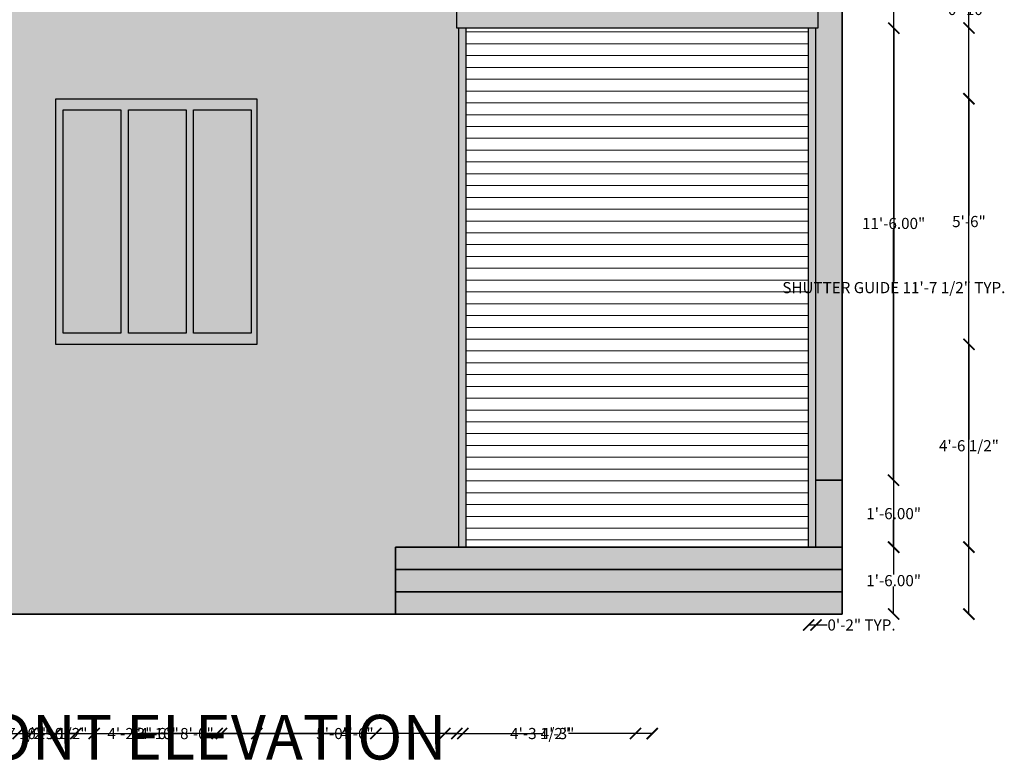
# Model space of a CAD drawing. Units: inches. Extents: x -654 to 390, y -40 to 648.
# Tile 4 of 13: x 126 to 390, y -40 to 159. Entities that reach past the tile are written whole.
import ezdxf

# ---------------------------------------------------------------- set-up
doc = ezdxf.new("R2010")
doc.units = ezdxf.units.IN
doc.header["$PDMODE"] = 3
for name, color, linetype, lineweight in [('A-ANNO-DIMS', 2, 'Continuous', 18), ('A-ANNO-TEXT', 7, 'Continuous', 25), ('A-DOOR', 3, 'Continuous', 25), ('A-ELEV', 7, 'Continuous', 35), ('A-ELEV-FILL', 252, 'Continuous', 13), ('A-ELEV-PATT', 8, 'Continuous', 13), ('A-GLAZ', 4, 'Continuous', 25)]:
    doc.layers.add(name, color=color, linetype=linetype, lineweight=lineweight)
doc.styles.get("Standard").update_dxf_attribs({"font": 'arial.ttf'})
doc.dimstyles.get("Standard").update_dxf_attribs({"dimtxt": 3, "dimasz": 3, "dimexe": 0.18, "dimexo": 0.0625, "dimgap": 0.09, "dimtad": 0, "dimtih": 1, "dimtoh": 1, "dimzin": 0, "dimdsep": 46, "dimlunit": 3, "dimtxsty": 'Standard', "dimblk": 'ARCHTICK', "dimcen": 0.09, "dimse1": 1, "dimse2": 1, "dimadec": 0, "dimazin": 0, "dimtfac": 1, "dimtofl": 0, "dimtmove": 0, "dimatfit": 3, "dimfxl": 1, "dimtolj": 1, "dimtzin": 0, "dimarcsym": 0})

# ---------------------------------------------------------------- blocks, each defined once
blk = doc.blocks.new('_ArchTick')
at = {"color": 0, "linetype": 'ByBlock', "const_width": 0.15}
blk.add_lwpolyline([(-0.5, -0.5), (0.5, 0.5)], dxfattribs=at)
blk = doc.blocks.new('*D2')
at = {"layer": 'A-ANNO-DIMS', "color": 0, "lineweight": -2, "transparency": 16777216}
for p, q in [((360.51, 17.13), (360.51, 9.76)), ((360.51, -0.87), (360.51, 6.51))]:
    blk.add_line(p, q, dxfattribs=at)
at = {"layer": 'Defpoints', "color": 0, "transparency": 16777216}
for p in [(346.65, 17.13), (360.51, 17.13), (346.65, -0.87)]:
    blk.add_point(p, dxfattribs=at)
at = {"layer": 'A-ANNO-DIMS', "color": 0, "lineweight": -2, "transparency": 16777216, "xscale": 3, "yscale": 3, "zscale": 3}
for p, rotation in [((360.51, 17.13), 90), ((360.51, -0.87), 270)]:
    blk.add_blockref('_ArchTick', p, dxfattribs=dict(at, rotation=rotation))
at = {"layer": 'A-ANNO-DIMS', "color": 0, "transparency": 16777216, "insert": (360.51, 8.13), "char_height": 3, "attachment_point": 5}
blk.add_mtext('\\A1;1\'-6.00"', dxfattribs=at)
blk = doc.blocks.new('*D3')
at = {"layer": 'A-ANNO-DIMS', "color": 0, "lineweight": -2, "transparency": 16777216}
for p, q in [((360.51, 35.13), (360.51, 27.76)), ((360.51, 17.13), (360.51, 24.51))]:
    blk.add_line(p, q, dxfattribs=at)
at = {"layer": 'Defpoints', "color": 0, "transparency": 16777216}
for p in [(346.65, 35.13), (360.51, 35.13), (346.65, 17.13)]:
    blk.add_point(p, dxfattribs=at)
at = {"layer": 'A-ANNO-DIMS', "color": 0, "lineweight": -2, "transparency": 16777216, "xscale": 3, "yscale": 3, "zscale": 3}
for p, rotation in [((360.51, 35.13), 90), ((360.51, 17.13), 270)]:
    blk.add_blockref('_ArchTick', p, dxfattribs=dict(at, rotation=rotation))
at = {"layer": 'A-ANNO-DIMS', "color": 0, "transparency": 16777216, "insert": (360.51, 26.13), "char_height": 3, "attachment_point": 5}
blk.add_mtext('\\A1;1\'-6.00"', dxfattribs=at)
blk = doc.blocks.new('*D4')
at = {"layer": 'A-ANNO-DIMS', "color": 0, "lineweight": -2, "transparency": 16777216}
for p, q in [((360.51, 173.13), (360.51, 105.76)), ((360.51, 35.13), (360.51, 102.51))]:
    blk.add_line(p, q, dxfattribs=at)
at = {"layer": 'Defpoints', "color": 0, "transparency": 16777216}
for p in [(346.65, 173.13), (360.51, 173.13), (346.65, 35.13)]:
    blk.add_point(p, dxfattribs=at)
at = {"layer": 'A-ANNO-DIMS', "color": 0, "lineweight": -2, "transparency": 16777216, "xscale": 3, "yscale": 3, "zscale": 3}
for p, rotation in [((360.51, 173.13), 90), ((360.51, 35.13), 270)]:
    blk.add_blockref('_ArchTick', p, dxfattribs=dict(at, rotation=rotation))
at = {"layer": 'A-ANNO-DIMS', "color": 0, "transparency": 16777216, "insert": (360.51, 104.13), "char_height": 3, "attachment_point": 5}
blk.add_mtext('\\A1;11\'-6.00"', dxfattribs=at)
blk = doc.blocks.new('SHUTTER-GUIDE')
for p, q in [((0, 0), (0, 139.5)), ((2, 0), (2, 139.5)), ((0, 0), (2, 0))]:
    blk.add_line(p, q)
blk = doc.blocks.new('*D73')
at = {"layer": 'A-ANNO-DIMS', "color": 0, "lineweight": -2, "transparency": 16777216}
for p, q in [((360.57, 156.63), (360.57, 88.52)), ((360.57, 17.13), (360.57, 85.24))]:
    blk.add_line(p, q, dxfattribs=at)
at = {"layer": 'Defpoints', "color": 0, "transparency": 16777216}
for p in [(339.65, 156.63), (360.57, 156.63), (339.65, 17.13)]:
    blk.add_point(p, dxfattribs=at)
at = {"layer": 'A-ANNO-DIMS', "color": 0, "lineweight": -2, "transparency": 16777216, "xscale": 3, "yscale": 3, "zscale": 3}
for p, rotation in [((360.57, 156.63), 90), ((360.57, 17.13), 270)]:
    blk.add_blockref('_ArchTick', p, dxfattribs=dict(at, rotation=rotation))
at = {"layer": 'A-ANNO-DIMS', "color": 0, "transparency": 16777216, "insert": (360.57, 86.88), "char_height": 3, "attachment_point": 5}
blk.add_mtext('\\A1;SHUTTER GUIDE 11\'-7 1/2" TYP.', dxfattribs=at)
blk = doc.blocks.new('*D74')
at = {"layer": 'A-ANNO-DIMS', "color": 0, "lineweight": -2, "transparency": 16777216}
for p, q in [((337.65, -3.79), (339.65, -3.79)), ((339.65, -3.79), (342.65, -3.79))]:
    blk.add_line(p, q, dxfattribs=at)
at = {"layer": 'Defpoints', "color": 0, "transparency": 16777216}
for p in [(337.65, 17.13), (339.65, 17.13), (339.65, -3.79)]:
    blk.add_point(p, dxfattribs=at)
at = {"layer": 'A-ANNO-DIMS', "color": 0, "lineweight": -2, "transparency": 16777216, "xscale": 3, "yscale": 3, "zscale": 3, "rotation": 180}
blk.add_blockref('_ArchTick', (337.65, -3.79), dxfattribs=at)
at = {"layer": 'A-ANNO-DIMS', "color": 0, "lineweight": -2, "transparency": 16777216, "xscale": 3, "yscale": 3, "zscale": 3}
blk.add_blockref('_ArchTick', (339.65, -3.79), dxfattribs=at)
at = {"layer": 'A-ANNO-DIMS', "color": 0, "transparency": 16777216, "insert": (351.88, -3.79), "char_height": 3, "attachment_point": 5}
blk.add_mtext('\\A1;0\'-2" TYP.', dxfattribs=at)
blk = doc.blocks.new('*D76')
at = {"layer": 'A-ANNO-DIMS', "color": 0, "lineweight": -2, "transparency": 16777216}
for p, q in [((380.75, 611.13), (380.75, 306.76)), ((380.75, -0.87), (380.75, 303.51))]:
    blk.add_line(p, q, dxfattribs=at)
at = {"layer": 'Defpoints', "color": 0, "transparency": 16777216}
for p in [(126.65, 611.13), (380.75, 611.13), (346.65, -0.87)]:
    blk.add_point(p, dxfattribs=at)
at = {"layer": 'A-ANNO-DIMS', "color": 0, "lineweight": -2, "transparency": 16777216, "xscale": 3, "yscale": 3, "zscale": 3}
for p, rotation in [((380.75, 611.13), 90), ((380.75, -0.87), 270)]:
    blk.add_blockref('_ArchTick', p, dxfattribs=dict(at, rotation=rotation))
at = {"layer": 'A-ANNO-DIMS', "color": 0, "transparency": 16777216, "insert": (380.75, 305.13), "char_height": 3, "attachment_point": 5}
blk.add_mtext('\\A1;51\'-0"', dxfattribs=at)
blk = doc.blocks.new('*D84')
at = {"layer": 'A-ANNO-DIMS', "color": 0, "lineweight": -2, "transparency": 16777216}
for p, q in [((115.65, -32.97), (118.07, -32.97)), ((135.36, -32.97), (132.94, -32.97))]:
    blk.add_line(p, q, dxfattribs=at)
at = {"layer": 'Defpoints', "color": 0, "transparency": 16777216}
for p in [(115.65, 83.13), (135.36, 71.63), (135.36, -32.97)]:
    blk.add_point(p, dxfattribs=at)
at = {"layer": 'A-ANNO-DIMS', "color": 0, "lineweight": -2, "transparency": 16777216, "xscale": 3, "yscale": 3, "zscale": 3, "rotation": 180}
blk.add_blockref('_ArchTick', (115.65, -32.97), dxfattribs=at)
at = {"layer": 'A-ANNO-DIMS', "color": 0, "lineweight": -2, "transparency": 16777216, "xscale": 3, "yscale": 3, "zscale": 3}
blk.add_blockref('_ArchTick', (135.36, -32.97), dxfattribs=at)
at = {"layer": 'A-ANNO-DIMS', "color": 0, "transparency": 16777216, "insert": (125.5, -32.97), "char_height": 3, "attachment_point": 5}
blk.add_mtext('\\A1;1\'-7 1/2"', dxfattribs=at)
blk = doc.blocks.new('*D85')
at = {"layer": 'A-ANNO-DIMS', "color": 0, "lineweight": -2, "transparency": 16777216}
for p, q in [((135.36, -32.97), (158.22, -32.97)), ((189.36, -32.97), (166.5, -32.97))]:
    blk.add_line(p, q, dxfattribs=at)
at = {"layer": 'Defpoints', "color": 0, "transparency": 16777216}
for p in [(135.36, 71.63), (189.36, 71.63), (189.36, -32.97)]:
    blk.add_point(p, dxfattribs=at)
at = {"layer": 'A-ANNO-DIMS', "color": 0, "lineweight": -2, "transparency": 16777216, "xscale": 3, "yscale": 3, "zscale": 3, "rotation": 180}
blk.add_blockref('_ArchTick', (135.36, -32.97), dxfattribs=at)
at = {"layer": 'A-ANNO-DIMS', "color": 0, "lineweight": -2, "transparency": 16777216, "xscale": 3, "yscale": 3, "zscale": 3}
blk.add_blockref('_ArchTick', (189.36, -32.97), dxfattribs=at)
at = {"layer": 'A-ANNO-DIMS', "color": 0, "transparency": 16777216, "insert": (162.36, -32.97), "char_height": 3, "attachment_point": 5}
blk.add_mtext('\\A1;4\'-6"', dxfattribs=at)
blk = doc.blocks.new('*D86')
at = {"layer": 'A-ANNO-DIMS', "color": 0, "lineweight": -2, "transparency": 16777216}
for p, q in [((380.75, 137.63), (380.75, 106.25)), ((380.75, 71.63), (380.75, 103.01))]:
    blk.add_line(p, q, dxfattribs=at)
at = {"layer": 'Defpoints', "color": 0, "transparency": 16777216}
for p in [(189.36, 137.63), (380.75, 137.63), (189.36, 71.63)]:
    blk.add_point(p, dxfattribs=at)
at = {"layer": 'A-ANNO-DIMS', "color": 0, "lineweight": -2, "transparency": 16777216, "xscale": 3, "yscale": 3, "zscale": 3}
for p, rotation in [((380.75, 137.63), 90), ((380.75, 71.63), 270)]:
    blk.add_blockref('_ArchTick', p, dxfattribs=dict(at, rotation=rotation))
at = {"layer": 'A-ANNO-DIMS', "color": 0, "transparency": 16777216, "insert": (380.75, 104.63), "char_height": 3, "attachment_point": 5}
blk.add_mtext('\\A1;5\'-6"', dxfattribs=at)
blk = doc.blocks.new('*D87')
at = {"layer": 'A-ANNO-DIMS', "color": 0, "lineweight": -2, "transparency": 16777216}
for p, q in [((380.75, 71.63), (380.75, 46.02)), ((380.75, 17.13), (380.75, 42.74))]:
    blk.add_line(p, q, dxfattribs=at)
at = {"layer": 'Defpoints', "color": 0, "transparency": 16777216}
for p in [(189.36, 71.63), (226.65, 17.13), (380.75, 17.13)]:
    blk.add_point(p, dxfattribs=at)
at = {"layer": 'A-ANNO-DIMS', "color": 0, "lineweight": -2, "transparency": 16777216, "xscale": 3, "yscale": 3, "zscale": 3}
for p, rotation in [((380.75, 71.63), 90), ((380.75, 17.13), 270)]:
    blk.add_blockref('_ArchTick', p, dxfattribs=dict(at, rotation=rotation))
at = {"layer": 'A-ANNO-DIMS', "color": 0, "transparency": 16777216, "insert": (380.75, 44.38), "char_height": 3, "attachment_point": 5}
blk.add_mtext('\\A1;4\'-6 1/2"', dxfattribs=at)
blk = doc.blocks.new('*D88')
at = {"layer": 'A-ANNO-DIMS', "color": 0, "lineweight": -2, "transparency": 16777216}
for p, q in [((189.36, -32.97), (212.12, -32.97)), ((243.15, -32.97), (220.39, -32.97))]:
    blk.add_line(p, q, dxfattribs=at)
at = {"layer": 'Defpoints', "color": 0, "transparency": 16777216}
for p in [(243.15, 156.63), (189.36, 137.63), (243.15, -32.97)]:
    blk.add_point(p, dxfattribs=at)
at = {"layer": 'A-ANNO-DIMS', "color": 0, "lineweight": -2, "transparency": 16777216, "xscale": 3, "yscale": 3, "zscale": 3, "rotation": 180}
blk.add_blockref('_ArchTick', (189.36, -32.97), dxfattribs=at)
at = {"layer": 'A-ANNO-DIMS', "color": 0, "lineweight": -2, "transparency": 16777216, "xscale": 3, "yscale": 3, "zscale": 3}
blk.add_blockref('_ArchTick', (243.15, -32.97), dxfattribs=at)
at = {"layer": 'A-ANNO-DIMS', "color": 0, "transparency": 16777216, "insert": (216.25, -32.97), "char_height": 3, "attachment_point": 5}
blk.add_mtext('\\A1;4\'-6"', dxfattribs=at)
blk = doc.blocks.new('*D89')
at = {"layer": 'A-ANNO-DIMS', "color": 0, "lineweight": -2, "transparency": 16777216}
for p, q in [((243.65, 643.23), (287.57, 643.23)), ((339.65, 643.23), (295.73, 643.23))]:
    blk.add_line(p, q, dxfattribs=at)
at = {"layer": 'Defpoints', "color": 0, "transparency": 16777216}
for p in [(339.65, 643.23), (243.65, 17.13), (339.65, 17.13)]:
    blk.add_point(p, dxfattribs=at)
at = {"layer": 'A-ANNO-DIMS', "color": 0, "lineweight": -2, "transparency": 16777216, "xscale": 3, "yscale": 3, "zscale": 3, "rotation": 180}
blk.add_blockref('_ArchTick', (243.65, 643.23), dxfattribs=at)
at = {"layer": 'A-ANNO-DIMS', "color": 0, "lineweight": -2, "transparency": 16777216, "xscale": 3, "yscale": 3, "zscale": 3}
blk.add_blockref('_ArchTick', (339.65, 643.23), dxfattribs=at)
at = {"layer": 'A-ANNO-DIMS', "color": 0, "transparency": 16777216, "insert": (291.65, 643.23), "char_height": 3, "attachment_point": 5}
blk.add_mtext('\\A1;8\'-0"', dxfattribs=at)
blk = doc.blocks.new('*D90')
at = {"layer": 'A-ANNO-DIMS', "color": 0, "lineweight": -2, "transparency": 16777216}
for p, q in [((339.65, 643.23), (346.65, 643.23)), ((346.65, 643.23), (349.65, 643.23))]:
    blk.add_line(p, q, dxfattribs=at)
at = {"layer": 'Defpoints', "color": 0, "transparency": 16777216}
for p in [(346.65, 643.23), (339.65, 17.13), (346.65, 17.13)]:
    blk.add_point(p, dxfattribs=at)
at = {"layer": 'A-ANNO-DIMS', "color": 0, "lineweight": -2, "transparency": 16777216, "xscale": 3, "yscale": 3, "zscale": 3, "rotation": 180}
blk.add_blockref('_ArchTick', (339.65, 643.23), dxfattribs=at)
at = {"layer": 'A-ANNO-DIMS', "color": 0, "lineweight": -2, "transparency": 16777216, "xscale": 3, "yscale": 3, "zscale": 3}
blk.add_blockref('_ArchTick', (346.65, 643.23), dxfattribs=at)
at = {"layer": 'A-ANNO-DIMS', "color": 0, "transparency": 16777216, "insert": (353.72, 643.23), "char_height": 3, "attachment_point": 5}
blk.add_mtext('\\A1;0\'-7"', dxfattribs=at)
blk = doc.blocks.new('*D91')
at = {"layer": 'A-ANNO-DIMS', "color": 0, "lineweight": -2, "transparency": 16777216}
for p, q in [((380.75, 166.63), (380.75, 163.26)), ((380.75, 156.63), (380.75, 160.01))]:
    blk.add_line(p, q, dxfattribs=at)
at = {"layer": 'Defpoints', "color": 0, "transparency": 16777216}
for p in [(243.15, 166.63), (380.75, 166.63), (243.15, 156.63)]:
    blk.add_point(p, dxfattribs=at)
at = {"layer": 'A-ANNO-DIMS', "color": 0, "lineweight": -2, "transparency": 16777216, "xscale": 3, "yscale": 3, "zscale": 3}
for p, rotation in [((380.75, 166.63), 90), ((380.75, 156.63), 270)]:
    blk.add_blockref('_ArchTick', p, dxfattribs=dict(at, rotation=rotation))
at = {"layer": 'A-ANNO-DIMS', "color": 0, "transparency": 16777216, "insert": (380.75, 161.63), "char_height": 3, "attachment_point": 5}
blk.add_mtext('\\A1;0\'-10"', dxfattribs=at)
blk = doc.blocks.new('*D92')
at = {"layer": 'A-ANNO-DIMS', "color": 0, "lineweight": -2, "transparency": 16777216}
for p, q in [((115.65, -32.97), (125.23, -32.97)), ((125.23, -32.97), (128.23, -32.97))]:
    blk.add_line(p, q, dxfattribs=at)
at = {"layer": 'Defpoints', "color": 0, "transparency": 16777216}
for p in [(115.65, 305.63), (125.23, 271.79), (125.23, -32.97)]:
    blk.add_point(p, dxfattribs=at)
at = {"layer": 'A-ANNO-DIMS', "color": 0, "lineweight": -2, "transparency": 16777216, "xscale": 3, "yscale": 3, "zscale": 3, "rotation": 180}
blk.add_blockref('_ArchTick', (115.65, -32.97), dxfattribs=at)
at = {"layer": 'A-ANNO-DIMS', "color": 0, "lineweight": -2, "transparency": 16777216, "xscale": 3, "yscale": 3, "zscale": 3}
blk.add_blockref('_ArchTick', (125.23, -32.97), dxfattribs=at)
at = {"layer": 'A-ANNO-DIMS', "color": 0, "transparency": 16777216, "insert": (135.8, -32.97), "char_height": 3, "attachment_point": 5}
blk.add_mtext('\\A1;0\'-9 1/2"', dxfattribs=at)
blk = doc.blocks.new('*D93')
at = {"layer": 'A-ANNO-DIMS', "color": 0, "lineweight": -2, "transparency": 16777216}
for p, q in [((125.23, -32.97), (169.2, -32.97)), ((221.33, -32.97), (177.36, -32.97))]:
    blk.add_line(p, q, dxfattribs=at)
at = {"layer": 'Defpoints', "color": 0, "transparency": 16777216}
for p in [(125.23, 271.79), (221.33, 271.79), (221.33, -32.97)]:
    blk.add_point(p, dxfattribs=at)
at = {"layer": 'A-ANNO-DIMS', "color": 0, "lineweight": -2, "transparency": 16777216, "xscale": 3, "yscale": 3, "zscale": 3, "rotation": 180}
blk.add_blockref('_ArchTick', (125.23, -32.97), dxfattribs=at)
at = {"layer": 'A-ANNO-DIMS', "color": 0, "lineweight": -2, "transparency": 16777216, "xscale": 3, "yscale": 3, "zscale": 3}
blk.add_blockref('_ArchTick', (221.33, -32.97), dxfattribs=at)
at = {"layer": 'A-ANNO-DIMS', "color": 0, "transparency": 16777216, "insert": (173.28, -32.97), "char_height": 3, "attachment_point": 5}
blk.add_mtext('\\A1;8\'-0"', dxfattribs=at)
blk = doc.blocks.new('*D95')
at = {"layer": 'A-ANNO-DIMS', "color": 0, "lineweight": -2, "transparency": 16777216}
for p, q in [((244.73, -32.97), (266.05, -32.97)), ((295.65, -32.97), (274.32, -32.97))]:
    blk.add_line(p, q, dxfattribs=at)
at = {"layer": 'Defpoints', "color": 0, "transparency": 16777216}
for p in [(244.73, 271.79), (295.65, 271.79), (295.65, -32.97)]:
    blk.add_point(p, dxfattribs=at)
at = {"layer": 'A-ANNO-DIMS', "color": 0, "lineweight": -2, "transparency": 16777216, "xscale": 3, "yscale": 3, "zscale": 3, "rotation": 180}
blk.add_blockref('_ArchTick', (244.73, -32.97), dxfattribs=at)
at = {"layer": 'A-ANNO-DIMS', "color": 0, "lineweight": -2, "transparency": 16777216, "xscale": 3, "yscale": 3, "zscale": 3}
blk.add_blockref('_ArchTick', (295.65, -32.97), dxfattribs=at)
at = {"layer": 'A-ANNO-DIMS', "color": 0, "transparency": 16777216, "insert": (270.19, -32.97), "char_height": 3, "attachment_point": 5}
blk.add_mtext('\\A1;4\'-3"', dxfattribs=at)
blk = doc.blocks.new('*D97')
at = {"layer": 'A-ANNO-DIMS', "color": 0, "lineweight": -2, "transparency": 16777216}
for p, q in [((128.74, -32.97), (130.81, -32.97)), ((140.74, -32.97), (138.68, -32.97))]:
    blk.add_line(p, q, dxfattribs=at)
at = {"layer": 'Defpoints', "color": 0, "transparency": 16777216}
for p in [(128.74, 173.13), (140.74, 173.13), (140.74, -32.97)]:
    blk.add_point(p, dxfattribs=at)
at = {"layer": 'A-ANNO-DIMS', "color": 0, "lineweight": -2, "transparency": 16777216, "xscale": 3, "yscale": 3, "zscale": 3, "rotation": 180}
blk.add_blockref('_ArchTick', (128.74, -32.97), dxfattribs=at)
at = {"layer": 'A-ANNO-DIMS', "color": 0, "lineweight": -2, "transparency": 16777216, "xscale": 3, "yscale": 3, "zscale": 3}
blk.add_blockref('_ArchTick', (140.74, -32.97), dxfattribs=at)
at = {"layer": 'A-ANNO-DIMS', "color": 0, "transparency": 16777216, "insert": (134.74, -32.97), "char_height": 3, "attachment_point": 5}
blk.add_mtext('\\A1;1\'-0"', dxfattribs=at)
blk = doc.blocks.new('*D98')
at = {"layer": 'A-ANNO-DIMS', "color": 0, "lineweight": -2, "transparency": 16777216}
for p, q in [((128.74, -32.97), (149.6, -32.97)), ((178.74, -32.97), (157.88, -32.97))]:
    blk.add_line(p, q, dxfattribs=at)
at = {"layer": 'Defpoints', "color": 0, "transparency": 16777216}
for p in [(128.74, 173.13), (178.74, 173.13), (178.74, -32.97)]:
    blk.add_point(p, dxfattribs=at)
at = {"layer": 'A-ANNO-DIMS', "color": 0, "lineweight": -2, "transparency": 16777216, "xscale": 3, "yscale": 3, "zscale": 3, "rotation": 180}
blk.add_blockref('_ArchTick', (128.74, -32.97), dxfattribs=at)
at = {"layer": 'A-ANNO-DIMS', "color": 0, "lineweight": -2, "transparency": 16777216, "xscale": 3, "yscale": 3, "zscale": 3}
blk.add_blockref('_ArchTick', (178.74, -32.97), dxfattribs=at)
at = {"layer": 'A-ANNO-DIMS', "color": 0, "transparency": 16777216, "insert": (153.74, -32.97), "char_height": 3, "attachment_point": 5}
blk.add_mtext('\\A1;4\'-2"', dxfattribs=at)
blk = doc.blocks.new('*D100')
at = {"layer": 'A-ANNO-DIMS', "color": 0, "lineweight": -2, "transparency": 16777216}
for p, q in [((145.65, -32.97), (157.49, -32.97)), ((179.88, -32.97), (168.03, -32.97))]:
    blk.add_line(p, q, dxfattribs=at)
at = {"layer": 'Defpoints', "color": 0, "transparency": 16777216}
for p in [(145.65, 355.63), (179.88, 355.63), (179.88, -32.97)]:
    blk.add_point(p, dxfattribs=at)
at = {"layer": 'A-ANNO-DIMS', "color": 0, "lineweight": -2, "transparency": 16777216, "xscale": 3, "yscale": 3, "zscale": 3, "rotation": 180}
blk.add_blockref('_ArchTick', (145.65, -32.97), dxfattribs=at)
at = {"layer": 'A-ANNO-DIMS', "color": 0, "lineweight": -2, "transparency": 16777216, "xscale": 3, "yscale": 3, "zscale": 3}
blk.add_blockref('_ArchTick', (179.88, -32.97), dxfattribs=at)
at = {"layer": 'A-ANNO-DIMS', "color": 0, "transparency": 16777216, "insert": (162.76, -32.97), "char_height": 3, "attachment_point": 5}
blk.add_mtext('\\A1;2\'-10"', dxfattribs=at)
blk = doc.blocks.new('*D102')
at = {"layer": 'A-ANNO-DIMS', "color": 0, "lineweight": -2, "transparency": 16777216}
for p, q in [((179.88, -32.97), (205.8, -32.97)), ((239.87, -32.97), (213.95, -32.97))]:
    blk.add_line(p, q, dxfattribs=at)
at = {"layer": 'Defpoints', "color": 0, "transparency": 16777216}
for p in [(179.88, 355.63), (239.87, 355.63), (239.87, -32.97)]:
    blk.add_point(p, dxfattribs=at)
at = {"layer": 'A-ANNO-DIMS', "color": 0, "lineweight": -2, "transparency": 16777216, "xscale": 3, "yscale": 3, "zscale": 3, "rotation": 180}
blk.add_blockref('_ArchTick', (179.88, -32.97), dxfattribs=at)
at = {"layer": 'A-ANNO-DIMS', "color": 0, "lineweight": -2, "transparency": 16777216, "xscale": 3, "yscale": 3, "zscale": 3}
blk.add_blockref('_ArchTick', (239.87, -32.97), dxfattribs=at)
at = {"layer": 'A-ANNO-DIMS', "color": 0, "transparency": 16777216, "insert": (209.87, -32.97), "char_height": 3, "attachment_point": 5}
blk.add_mtext('\\A1;5\'-0"', dxfattribs=at)
blk = doc.blocks.new('*D103')
at = {"layer": 'A-ANNO-DIMS', "color": 0, "lineweight": -2, "transparency": 16777216}
for p, q in [((239.87, -32.97), (257.87, -32.97)), ((291.14, -32.97), (273.14, -32.97))]:
    blk.add_line(p, q, dxfattribs=at)
at = {"layer": 'Defpoints', "color": 0, "transparency": 16777216}
for p in [(239.87, 355.63), (291.14, 355.63), (291.14, -32.97)]:
    blk.add_point(p, dxfattribs=at)
at = {"layer": 'A-ANNO-DIMS', "color": 0, "lineweight": -2, "transparency": 16777216, "xscale": 3, "yscale": 3, "zscale": 3, "rotation": 180}
blk.add_blockref('_ArchTick', (239.87, -32.97), dxfattribs=at)
at = {"layer": 'A-ANNO-DIMS', "color": 0, "lineweight": -2, "transparency": 16777216, "xscale": 3, "yscale": 3, "zscale": 3}
blk.add_blockref('_ArchTick', (291.14, -32.97), dxfattribs=at)
at = {"layer": 'A-ANNO-DIMS', "color": 0, "transparency": 16777216, "insert": (265.51, -32.97), "char_height": 3, "attachment_point": 5}
blk.add_mtext('\\A1;4\'-3 1/2"', dxfattribs=at)

msp = doc.modelspace()

# ---------------------------------------------------------------- hatches: boundary and pattern name
at = {"layer": 'A-ELEV-FILL'}
h = msp.add_hatch(color=256, dxfattribs=at)
h.dxf.hatch_style = 1
h.paths.add_polyline_path([(138.646, 438.634), (107.646, 438.634), (107.646, 359.634), (138.646, 359.634)])
h.paths.add_polyline_path([(136.646, 436.634), (136.646, 361.634), (109.646, 361.634), (109.646, 436.634)], flags=16)
h.paths.add_polyline_path([(179.877, 410.786), (145.646, 410.786), (145.646, 407.786), (153.285, 407.786), (153.285, 357.634), (145.646, 357.634), (145.646, 355.634), (179.877, 355.634)])
h.paths.add_polyline_path([(178.123, 407.786), (178.123, 357.634), (155.286, 357.634), (155.286, 407.786)], flags=16)
h.paths.add_polyline_path([(291.141, 410.786), (239.871, 410.786), (239.871, 355.634), (241.996, 355.634), (241.996, 407.786), (269.317, 407.786), (269.317, 355.634), (271.318, 355.634), (271.318, 407.786), (289.369, 407.786), (289.369, 355.634), (291.141, 355.634)])
h.paths.add_polyline_path([(128.225, 268.786), (128.742, 268.786), (128.742, 271.786), (125.225, 271.786), (125.225, 216.634), (128.225, 216.634)])
h.paths.add_polyline_path([(140.742, 271.786), (130.742, 271.786), (130.742, 268.786), (140.742, 268.786)])
h.paths.add_polyline_path([(152.742, 271.786), (142.742, 271.786), (142.742, 268.786), (152.742, 268.786)])
h.paths.add_polyline_path([(164.742, 271.786), (154.742, 271.786), (154.742, 268.786), (164.742, 268.786)])
h.paths.add_polyline_path([(176.742, 271.786), (167.328, 271.786), (166.742, 271.786), (166.742, 268.786), (167.328, 268.786), (167.328, 216.634), (169.328, 216.634), (169.328, 268.786), (176.742, 268.786)])
h.paths.add_polyline_path([(221.328, 271.786), (178.742, 271.786), (178.742, 268.786), (184.828, 268.786), (184.828, 216.634), (186.829, 216.634), (186.829, 268.786), (202.329, 268.786), (202.329, 216.634), (204.325, 216.634), (204.325, 268.786), (219.825, 268.786), (219.825, 216.634), (221.328, 216.634)])
h.paths.add_polyline_path([(295.646, 271.786), (244.726, 271.786), (244.726, 216.634), (246.481, 216.634), (246.481, 268.786), (269.317, 268.786), (269.317, 216.634), (271.318, 216.634), (271.318, 268.786), (286.818, 268.786), (286.818, 216.634), (288.814, 216.634), (288.814, 268.786), (295.646, 268.786)])
h.paths.add_polyline_path([(295.646, 216.634), (178.742, 216.634), (178.742, 214.634), (295.646, 214.634)])
h.paths.add_polyline_path([(128.742, 216.634), (123.485, 216.634), (123.485, 214.634), (128.742, 214.634)])
h.paths.add_polyline_path([(140.742, 216.634), (130.742, 216.634), (130.742, 214.634), (140.742, 214.634)])
h.paths.add_polyline_path([(152.742, 216.634), (142.742, 216.634), (142.742, 214.634), (152.742, 214.634)])
h.paths.add_polyline_path([(164.742, 216.634), (154.742, 216.634), (154.742, 214.634), (164.742, 214.634)])
h.paths.add_polyline_path([(176.742, 216.634), (166.742, 216.634), (166.742, 214.634), (176.742, 214.634)])
h.paths.add_polyline_path([(128.742, 192.634), (119.386, 192.634), (119.386, 190.634), (128.742, 190.634)])
h.paths.add_polyline_path([(140.742, 192.634), (130.742, 192.634), (130.742, 190.634), (140.742, 190.634)])
h.paths.add_polyline_path([(152.742, 192.634), (142.742, 192.634), (142.742, 190.634), (152.742, 190.634)])
h.paths.add_polyline_path([(164.742, 192.634), (154.742, 192.634), (154.742, 190.634), (164.742, 190.634)])
h.paths.add_polyline_path([(176.742, 192.634), (166.742, 192.634), (166.742, 190.634), (176.742, 190.634)])
h.paths.add_polyline_path([(295.646, 192.634), (178.742, 192.634), (178.742, 190.634), (295.646, 190.634)])
h.paths.add_polyline_path([(189.362, 137.63), (135.362, 137.63), (135.362, 71.63), (189.362, 71.63)])
h.paths.add_polyline_path([(154.862, 134.63), (170.362, 134.63), (170.362, 74.63), (154.862, 74.63)], flags=16)
h.paths.add_polyline_path([(152.862, 134.63), (152.862, 74.63), (137.362, 74.63), (137.362, 134.63)], flags=16)
h.paths.add_polyline_path([(172.358, 134.63), (187.858, 134.63), (187.858, 74.63), (172.358, 74.63)], flags=16)
h.paths.add_polyline_path([(113.646, 83.134), (62.646, 83.134), (62.646, 17.134), (113.646, 17.134)])
h.paths.add_polyline_path([(96.484, 80.08), (109.984, 80.08), (109.984, 20.08), (96.484, 20.08)], flags=16)
h.paths.add_polyline_path([(93.843, 80.08), (93.843, 20.08), (80.343, 20.08), (80.343, 80.08)], flags=16)
h.paths.add_polyline_path([(78.051, 80.08), (78.051, 20.08), (64.551, 20.08), (64.551, 80.08)], flags=16)
h.paths.add_polyline_path([(60.646, 83.134), (9.646, 83.134), (9.646, 17.134), (60.646, 17.134)])
h.paths.add_polyline_path([(58.197, 80.08), (58.197, 20.08), (44.697, 20.08), (44.697, 80.08)], flags=16)
h.paths.add_polyline_path([(41.55, 80.08), (41.55, 20.08), (28.05, 20.08), (28.05, 80.08)], flags=16)
h.paths.add_polyline_path([(25.146, 80.08), (25.146, 20.08), (11.646, 20.08), (11.646, 80.08)], flags=16)
h.paths.add_polyline_path([(9.646, 83.134), (7.646, 83.134), (7.646, 73.776), (9.646, 73.776)])
h.paths.add_polyline_path([(9.646, 65.663), (7.646, 65.663), (7.646, 36.041), (9.646, 36.041)])
h.paths.add_polyline_path([(9.646, 27.928), (7.646, 27.928), (7.646, 17.134), (9.646, 17.134)])
h.paths.add_polyline_path([(115.646, 83.134), (113.646, 83.134), (113.646, 73.776), (115.646, 73.776)])
h.paths.add_polyline_path([(115.646, 65.663), (113.646, 65.663), (113.646, 35.502), (115.646, 35.502)])
h.paths.add_polyline_path([(115.646, 27.389), (113.646, 27.389), (113.646, 17.134), (115.646, 17.134)])
h.paths.add_polyline_path([(8.146, 89.642), (-1.854, 89.642), (-1.854, 87.642), (8.146, 87.642)])
h.paths.add_polyline_path([(245.646, 156.634), (243.646, 156.634), (243.646, 17.134), (245.646, 17.134)])
h.paths.add_polyline_path([(339.646, 156.634), (337.646, 156.634), (337.646, 17.134), (339.646, 17.134)])
h = msp.add_hatch(color=256, dxfattribs=at)
h.dxf.hatch_style = 1
h.paths.add_polyline_path([(243.646, 156.634), (243.146, 156.634), (243.146, 166.634), (340.146, 166.634), (340.146, 156.634), (339.646, 156.634), (339.646, 35.134), (346.646, 35.134), (346.646, 168.634), (115.646, 168.634), (115.646, 17.134), (118.646, 17.134), (118.646, -0.866), (226.646, -0.866), (226.646, 17.134), (243.646, 17.134)])
h.paths.add_polyline_path([(189.362, 71.63), (135.362, 71.63), (135.362, 137.63), (189.362, 137.63)], flags=16)
h.paths.add_polyline_path([(187.858, 74.63), (172.358, 74.63), (172.358, 134.63), (187.858, 134.63)], flags=0)
h.paths.add_polyline_path([(170.362, 74.63), (154.862, 74.63), (154.862, 134.63), (170.362, 134.63)], flags=0)
h.paths.add_polyline_path([(152.862, 74.63), (137.362, 74.63), (137.362, 134.63), (152.862, 134.63)], flags=0)
h.paths.add_polyline_path([(346.646, 35.134), (339.646, 35.134), (339.646, 17.134), (346.646, 17.134)], flags=17)
h = msp.add_hatch(color=256, dxfattribs=at)
h.dxf.hatch_style = 1
h.paths.add_polyline_path([(340.146, 166.634), (243.146, 166.634), (243.146, 156.634), (340.146, 156.634)])
h = msp.add_hatch(color=256, dxfattribs=at)
h.dxf.hatch_style = 1
h.paths.add_polyline_path([(346.646, 5.134), (226.646, 5.134), (226.646, -0.866), (346.646, -0.866)])
h.paths.add_polyline_path([(346.646, 11.134), (226.646, 11.134), (226.646, 5.134), (346.646, 5.134)])
h.paths.add_polyline_path([(346.646, 17.134), (226.646, 17.134), (226.646, 11.134), (346.646, 11.134)])
at = {"layer": 'A-ELEV-PATT'}
h = msp.add_hatch(dxfattribs=at)
h.set_pattern_fill('GOST_GLASS', color=256)
h.paths.add_polyline_path([(34.168, 540.134), (18.646, 540.134), (18.646, 494.634), (34.168, 494.634)])
h.paths.add_polyline_path([(50.651, 540.134), (35.875, 540.134), (35.875, 494.634), (50.651, 494.634)])
h.paths.add_polyline_path([(23.368, 492.634), (18.646, 492.634), (18.646, 482.634), (23.368, 482.634)])
h.paths.add_polyline_path([(30.384, 492.634), (24.368, 492.634), (24.368, 482.634), (30.384, 482.634)])
h.paths.add_polyline_path([(34.168, 492.634), (31.384, 492.634), (31.384, 482.634), (34.168, 482.634)])
h.paths.add_polyline_path([(44.416, 492.634), (38.4, 492.634), (38.4, 482.634), (44.416, 482.634)])
h.paths.add_polyline_path([(50.651, 492.634), (45.416, 492.634), (45.416, 482.634), (50.651, 482.634)])
h.paths.add_polyline_path([(37.4, 492.634), (35.875, 492.634), (35.875, 482.634), (37.4, 482.634)])
h.paths.add_polyline_path([(52.146, 408.134), (17.146, 408.134), (17.146, 360.234), (52.146, 360.234)])
h.paths.add_polyline_path([(52.146, 359.234), (17.146, 359.234), (17.146, 311.834), (52.146, 311.834)])
h.paths.add_polyline_path([(52.146, 310.834), (17.146, 310.834), (17.146, 263.434), (52.146, 263.434)])
h.paths.add_polyline_path([(52.146, 262.434), (17.146, 262.434), (17.146, 215.034), (52.146, 215.034)])
h.paths.add_polyline_path([(52.146, 214.034), (17.146, 214.034), (17.146, 166.134), (52.146, 166.134)])
h.paths.add_polyline_path([(44.556, 113.134), (33.082, 113.134), (33.082, 83.134), (44.556, 83.134)])
h.paths.add_polyline_path([(29.904, 113.134), (18.431, 113.134), (18.431, 83.134), (29.904, 83.134)])
h.paths.add_polyline_path([(59.143, 113.134), (47.67, 113.134), (47.67, 83.134), (59.143, 83.134)])
h.paths.add_polyline_path([(152.862, 134.63), (137.362, 134.63), (137.362, 74.63), (152.862, 74.63)])
h.paths.add_polyline_path([(170.362, 134.63), (154.862, 134.63), (154.862, 74.63), (170.362, 74.63)])
h.paths.add_polyline_path([(187.858, 134.63), (172.358, 134.63), (172.358, 74.63), (187.858, 74.63)])
h = msp.add_hatch(dxfattribs=at)
h.set_pattern_fill('LINE', color=256)
h.paths.add_polyline_path([(337.646, 156.634), (245.646, 156.634), (245.646, 17.134), (337.646, 17.134)])

# ---------------------------------------------------------------- linework, layer by layer
at = {"layer": 'A-DOOR'}
msp.add_lwpolyline([(243.146, 166.634), (340.146, 166.634), (340.146, 156.634), (243.146, 156.634)], close=True, dxfattribs=at)
at = {"layer": 'A-ELEV'}
for p, q in [((346.646, -0.866), (346.646, 587.634)), ((346.646, 17.134), (346.646, 173.134)), ((339.646, 35.134), (346.646, 35.134)), ((226.646, 17.134), (226.646, -0.866)), ((226.646, 17.134), (346.646, 17.134)), ((226.646, 11.134), (346.646, 11.134)), ((226.646, 5.134), (346.646, 5.134)), ((-1.354, -0.866), (346.646, -0.866))]:
    msp.add_line(p, q, dxfattribs=at)
at = {"layer": 'A-GLAZ'}
for points in [[(135.362, 137.63), (189.362, 137.63), (189.362, 71.63), (135.362, 71.63)], [(137.362, 134.63), (152.862, 134.63), (152.862, 74.63), (137.362, 74.63)], [(154.862, 134.63), (170.362, 134.63), (170.362, 74.63), (154.862, 74.63)], [(172.358, 134.63), (187.858, 134.63), (187.858, 74.63), (172.358, 74.63)]]:
    msp.add_lwpolyline(points, close=True, dxfattribs=at)

# ---------------------------------------------------------------- block references
at = {"layer": 'A-DOOR'}
for p in [(243.646, 17.134), (337.646, 17.134)]:
    msp.add_blockref('SHUTTER-GUIDE', p, dxfattribs=at)

# ---------------------------------------------------------------- texts
at = {"layer": 'A-ANNO-TEXT', "insert": (97.321, -7.947), "char_height": 12, "attachment_point": 1}
msp.add_mtext_dynamic_manual_height_columns('\\PFRONT ELEVATION', width=187.36466, gutter_width=12.5, heights=[0], dxfattribs=at)

# ---------------------------------------------------------------- dimensions: what is measured, and where the dimension line sits
at = {"layer": 'A-ANNO-DIMS'}
for base, p1, p2, picture, middle in [((339.646, 643.234), (243.646, 17.134), (339.646, 17.134), '*D89', (291.646, 643.234)), ((346.646, 643.234), (339.646, 17.134), (346.646, 17.134), '*D90', (353.724, 643.234)), ((179.877, -32.966), (145.646, 355.634), (179.877, 355.634), '*D100', (162.762, -32.966)), ((239.871, -32.966), (179.877, 355.634), (239.871, 355.634), '*D102', (209.874, -32.966)), ((291.141, -32.966), (239.871, 355.634), (291.141, 355.634), '*D103', (265.506, -32.966)), ((125.225, -32.966), (115.646, 305.634), (125.225, 271.786), '*D92', (135.798, -32.966)), ((221.328, -32.966), (125.225, 271.786), (221.328, 271.786), '*D93', (173.277, -32.966)), ((295.646, -32.966), (244.726, 271.786), (295.646, 271.786), '*D95', (270.186, -32.966)), ((140.742, -32.966), (128.742, 173.134), (140.742, 173.134), '*D97', (134.742, -32.966)), ((178.742, -32.966), (128.742, 173.134), (178.742, 173.134), '*D98', (153.742, -32.966)), ((243.146, -32.966), (189.362, 137.63), (243.146, 156.634), '*D88', (216.254, -32.966)), ((135.362, -32.966), (115.646, 83.134), (135.362, 71.63), '*D84', (125.504, -32.966)), ((189.362, -32.966), (135.362, 71.63), (189.362, 71.63), '*D85', (162.362, -32.966))]:
    dim = msp.add_linear_dim(base=base, p1=p1, p2=p2, dimstyle='Standard', override={"dimdec": 1, "dimlfac": 1, "dimrnd": 0, "dimzin": 1, "dimdsep": 46, "dimlunit": 4, "dimfrac": 2}, dxfattribs=at)
    dim.commit()
    dim.dimension.update_dxf_attribs({"geometry": picture, "text_midpoint": middle})
for base, p1, p2, override, picture, middle in [((380.746, 611.134), (346.646, -0.866), (126.646, 611.134), {"dimdec": 1, "dimlfac": 1, "dimrnd": 0, "dimzin": 1, "dimdsep": 46, "dimlunit": 4, "dimfrac": 2}, '*D76', (380.746, 305.134)), ((360.508, 173.134), (346.646, 35.134), (346.646, 173.134), {"dimclrd": 0, "dimclre": 0, "dimclrt": 0, "dimtmove": 1}, '*D4', (360.508, 104.134)), ((380.746, 166.634), (243.146, 156.634), (243.146, 166.634), {"dimdec": 1, "dimlfac": 1, "dimrnd": 0, "dimzin": 1, "dimdsep": 46, "dimlunit": 4, "dimfrac": 2}, '*D91', (380.746, 161.634)), ((380.746, 137.63), (189.362, 71.63), (189.362, 137.63), {"dimdec": 1, "dimlfac": 1, "dimrnd": 0, "dimzin": 1, "dimdsep": 46, "dimlunit": 4, "dimfrac": 2}, '*D86', (380.746, 104.63)), ((380.746, 17.134), (189.362, 71.63), (226.646, 17.134), {"dimdec": 1, "dimlfac": 1, "dimrnd": 0, "dimzin": 1, "dimdsep": 46, "dimlunit": 4, "dimfrac": 2}, '*D87', (380.746, 44.382)), ((360.508, 35.134), (346.646, 17.134), (346.646, 35.134), {"dimclrd": 0, "dimclre": 0, "dimclrt": 0, "dimtmove": 1}, '*D3', (360.508, 26.134)), ((360.508, 17.134), (346.646, -0.866), (346.646, 17.134), {"dimclrd": 0, "dimclre": 0, "dimclrt": 0}, '*D2', (360.508, 8.134))]:
    dim = msp.add_linear_dim(base=base, p1=p1, p2=p2, angle=90, dimstyle='Standard', override=override, dxfattribs=at)
    dim.commit()
    dim.dimension.update_dxf_attribs({"geometry": picture, "text_midpoint": middle})
dim = msp.add_linear_dim(base=(360.571, 156.634), p1=(339.646, 17.134), p2=(339.646, 156.634), angle=90, text='SHUTTER GUIDE <> TYP.', dimstyle='Standard', override={"dimdec": 1, "dimrnd": 0, "dimzin": 1, "dimlunit": 4, "dimfrac": 2}, dxfattribs=at)
dim.commit()
dim.dimension.update_dxf_attribs({"geometry": '*D73', "text_midpoint": (360.571, 86.884)})
dim = msp.add_linear_dim(base=(339.646, -3.791), p1=(337.646, 17.134), p2=(339.646, 17.134), text='<> TYP.', dimstyle='Standard', override={"dimdec": 1, "dimrnd": 0, "dimzin": 1, "dimlunit": 4, "dimfrac": 2}, dxfattribs=at)
dim.commit()
dim.dimension.update_dxf_attribs({"geometry": '*D74', "text_midpoint": (351.88, -3.791)})

doc.saveas('drawing.dxf')
